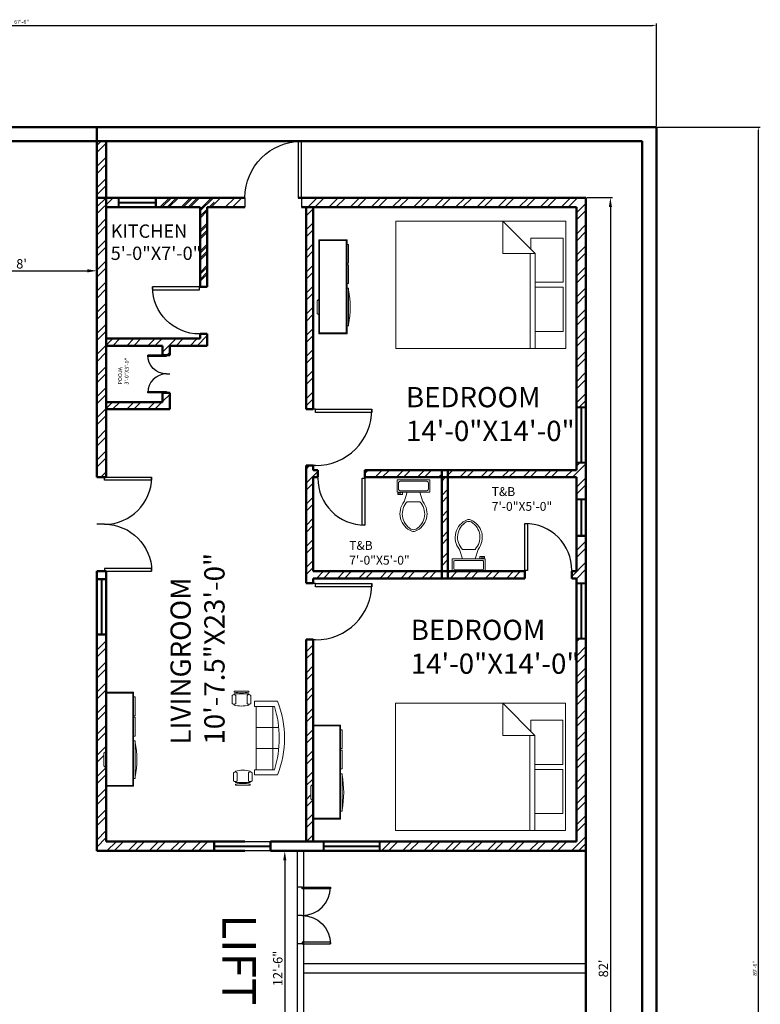
# Model space of a CAD drawing. Units: inches. Extents: x -12550 to 6516, y 1273 to 18700.
# Tile 15 of 19: x 4811 to 5284, y 1958 to 2587. Entities that reach past the tile are written whole.
import ezdxf

# ---------------------------------------------------------------- set-up
doc = ezdxf.new("R2010")
doc.units = ezdxf.units.IN
for name, color, linetype, lineweight in [('A-ANNO-DIMS', 2, 'Continuous', 18), ('A-AREA-IDEN', 1, 'Continuous', 18), ('A-DOOR', 5, 'Continuous', 25), ('A-EQPM', 4, 'Continuous', 25), ('A-FURN', 8, 'Continuous', 18), ('A-GLAZ', 3, 'Continuous', 25), ('A-WALL', 7, 'Continuous', 50), ('A-WALL-PATT', 8, 'Continuous', 13)]:
    doc.layers.add(name, color=color, linetype=linetype, lineweight=lineweight)
doc.styles.get("Standard").update_dxf_attribs({"font": 'arial.ttf'})
doc.dimstyles.new('ISO-25', dxfattribs={"dimtxt": 2.5, "dimasz": 2.5, "dimexe": 1.25, "dimexo": 0.625, "dimtad": 1, "dimlunit": 4, "dimtxsty": 'Standard', "dimcen": 2.5, "dimadec": 0, "dimazin": 0, "dimtfac": 1, "dimtmove": 0, "dimatfit": 3, "dimfxl": 1, "dimarcsym": 0})
pattern_1 = [(45, (2434.941, 0), (-6.735192, 6.735192), []), (45, (2439.432, 0), (-6.735192, 6.735192), [])]
pattern_2 = [(45, (2434.941, 567), (-6.735192, 6.735192), []), (45, (2439.432, 567), (-6.735192, 6.735192), [])]

# ---------------------------------------------------------------- blocks, each defined once
blk = doc.blocks.new('*U2')
for p, q in [((0, 0), (0, -5)), ((30, 0), (30, -5))]:
    blk.add_line(p, q)
blk.add_lwpolyline([(0, 0), (0, 30), (1.75, 30), (1.75, 0)], close=True)
blk.add_arc((0, 0), 30, 0, 90)
blk = doc.blocks.new('Bed - Queen')
for p, q in [((0, -80.00003), (0, 0)), ((0, 0), (59.99999, 0)), ((59.99999, 0), (59.99999, -80.00003)), ((7.99999, -1.2), (28.79998, -1.2)), ((7.99999, -14.4), (7.99999, -1.2)), ((28.79998, -1.2), (28.79998, -14.4)), ((31.19999, -1.2), (51.99999, -1.2)), ((31.19999, -14.4), (31.19999, -1.2)), ((51.99999, -1.2), (51.99999, -16.4)), ((0, -14.4), (44.8, -14.4)), ((44.8, -16.8), (0, -16.8)), ((59.99999, -29.6), (44.8, -14.4)), ((44.8, -14.4), (44.8, -29.6)), ((51.99999, -16.4), (46.79936, -16.4)), ((44.8, -29.6), (59.99999, -29.6)), ((59.99999, -80.00003), (0, -80.00003))]:
    blk.add_line(p, q)
blk = doc.blocks.new('Toilet - top')
for p, q in [((9.5, -6), (9.5, -2)), ((-10, -8.5), (-8, -8.5)), ((-10, -9.5), (-10, -8.5)), ((-7, -9.5), (-10, -9.5)), ((-8, -8.5), (-8, -8)), ((-7, -8), (-7, -9.5)), ((-4, -8), (-6, -14)), ((4, -8), (6, -14)), ((4, -14), (-4, -14))]:
    blk.add_line(p, q)
blk.add_lwpolyline([(10.5, -8), (10.5, 0), (-10.5, 0), (-10.5, -8)], close=True)
for points in [[(-9.5, -2), (-9.5, -6)], [(8.5, -1), (-8.5, -1)], [(-8.5, -7), (8.5, -7)]]:
    blk.add_lwpolyline(points)
for centre, radius, start, end in [((-8.62, -1.88), 0.884, 81.8699, 188.1301), ((-8.62, -6.12), 0.884, 171.8699, 278.1301), ((8.62, -1.88), 0.884, 351.8699, 98.1301), ((8.62, -6.12), 0.884, 261.8699, 8.1301), ((3.52, -21.58), 12.17, 141.46911, 247.97143), ((4.2, -21.82), 11.33, 136.36773, 238.94682), ((-3.52, -21.58), 12.17, 292.02843, 38.53071), ((-4.2, -21.82), 11.33, 301.05301, 43.63209), ((0, -27.88), 4, 245.73182, 294.26817), ((0, -29), 4, 254.86053, 285.13947)]:
    blk.add_arc(centre, radius, start, end)
blk = doc.blocks.new('Entertainment Center')
for p, q in [((-4, 0), (-5, -1)), ((4, 0), (-4, 0)), ((5, -1), (4, 0)), ((-17, -19), (-17, -1)), ((-17, -1), (43, -1)), ((-16.5, -18.5), (-16.5, -1.5)), ((-16.5, -1.5), (42.5, -1.5)), ((42.5, -1.5), (42.5, -18.5)), ((43, -1), (43, -19)), ((42.5, -18.5), (-16.5, -18.5)), ((43, -19), (-17, -19)), ((-12, -20), (-12, -19)), ((12, -20), (-12, -20)), ((12, -19), (12, -20)), ((15, -20), (15, -19)), ((27, -20), (15, -20)), ((27, -19), (27, -20)), ((28, -20), (28, -19)), ((40, -20), (28, -20)), ((40, -19), (40, -20))]:
    blk.add_line(p, q)
blk.add_arc((0, 40), 61, 259.6111, 280.3889)
blk = doc.blocks.new('Sofa - Roundback 7 ft.')
for p, q in [((-12.00002, -32.4421), (-12.00003, -6.5971)), ((11.99997, -32.4421), (11.99998, -6.5971)), ((-36.000027, -34), (-36.000027, -11.4696)), ((-35.999844, -13.3819), (35.9998, -13.3819)), ((35.99998, -34), (35.99998, -11.4696)), ((-36.000027, -32.4421), (35.99998, -32.4421))]:
    blk.add_line(p, q)
for points in [[(-36.000027, -34), (-42.000027, -34), (-42.000027, -8)], [(41.99998, -8), (41.99998, -34), (35.99998, -34)]]:
    blk.add_lwpolyline(points)
for centre, radius, start, end in [((0, -114.25), 114.25, 68.43141, 111.5686), ((-0.00001, -127.1968), 121.1968, 72.72033, 107.2797)]:
    blk.add_arc(centre, radius, start, end)
blk = doc.blocks.new('Chair - Desk')
for p, q in [((-8.5, 0), (-8.5, -1)), ((-8.5, 0), (8.5, 0)), ((8.5, 0), (8.5, -1)), ((-10.5, -5), (-10.5, -14)), ((-8.5, -3), (-8.5, -4)), ((-8.5, -3), (8.5, -3)), ((-6.5, -14), (-6.5, -5)), ((-2, -3), (-2, -1.9355)), ((2, -1.9576), (2, -3)), ((6.5, -5), (6.5, -14)), ((8.5, -3), (8.5, -4)), ((10.5, -14), (10.5, -5)), ((-8.5, -15), (-8.5, -16)), ((8.5, -15), (8.5, -16))]:
    blk.add_line(p, q)
for centre, radius, start, end in [((-8.5, -6.5), 2.5, 36.8699, 143.1301), ((0, 34.625), 36.625, 256.5803, 283.4197), ((8.5, -6.5), 2.5, 36.8699, 143.1301), ((-8.5, -12.5), 2.5, 216.8699, 323.1301), ((0, 19.625), 36.625, 256.5803, 283.4197), ((8.5, -12.5), 2.5, 216.8699, 323.1301)]:
    blk.add_arc(centre, radius, start, end)
blk = doc.blocks.new('*D40')
at = {"layer": 'A-ANNO-DIMS', "color": 0, "lineweight": -2, "transparency": 16777216}
for p, q in [((4988.01, 2056.25), (4979.29, 2056.25)), ((4980.54, 2050.25), (4980.54, 1912.25)), ((4988.01, 1906.25), (4979.29, 1906.25))]:
    blk.add_line(p, q, dxfattribs=at)
at = {"layer": 'A-ANNO-DIMS', "color": 0, "transparency": 16777216}
for points in [[(4979.54, 2050.25), (4981.54, 2050.25), (4980.54, 2056.25)], [(4979.54, 1912.25), (4981.54, 1912.25), (4980.54, 1906.25)]]:
    blk.add_solid(points, dxfattribs=at)
at = {"layer": 'Defpoints', "color": 0, "transparency": 16777216}
for p in [(4988.63, 2056.25), (4980.54, 1906.25), (4988.63, 1906.25)]:
    blk.add_point(p, dxfattribs=at)
at = {"layer": 'A-ANNO-DIMS', "color": 0, "transparency": 16777216, "insert": (4976.86, 1981.25), "char_height": 6, "attachment_point": 5, "rotation": 90}
blk.add_mtext('12\'-6"', dxfattribs=at)
blk = doc.blocks.new('*D42')
at = {"layer": 'A-ANNO-DIMS', "color": 0, "lineweight": -2, "transparency": 16777216}
for p, q in [((5173.26, 2473.25), (5189.5, 2473.25)), ((5188.25, 2467.25), (5188.25, 1495.25)), ((5173.26, 1489.25), (5189.5, 1489.25))]:
    blk.add_line(p, q, dxfattribs=at)
at = {"layer": 'A-ANNO-DIMS', "color": 0, "transparency": 16777216}
for points in [[(5187.25, 2467.25), (5189.25, 2467.25), (5188.25, 2473.25)], [(5187.25, 1495.25), (5189.25, 1495.25), (5188.25, 1489.25)]]:
    blk.add_solid(points, dxfattribs=at)
at = {"layer": 'Defpoints', "color": 0, "transparency": 16777216}
for p in [(5172.63, 2473.25), (5172.63, 1489.25), (5188.25, 1489.25)]:
    blk.add_point(p, dxfattribs=at)
at = {"layer": 'A-ANNO-DIMS', "color": 0, "transparency": 16777216, "insert": (5184.56, 1981.25), "char_height": 6, "attachment_point": 5, "rotation": 90}
blk.add_mtext("82'", dxfattribs=at)
blk = doc.blocks.new('*D39')
at = {"layer": 'A-ANNO-DIMS', "color": 0, "lineweight": -2, "transparency": 16777216}
for p, q in [((4764.63, 2407.12), (4764.63, 2427.81)), ((4770.63, 2426.56), (4854.63, 2426.56)), ((4860.63, 2407.12), (4860.63, 2427.81))]:
    blk.add_line(p, q, dxfattribs=at)
at = {"layer": 'A-ANNO-DIMS', "color": 0, "transparency": 16777216}
for points in [[(4770.63, 2427.56), (4770.63, 2425.56), (4764.63, 2426.56)], [(4854.63, 2427.56), (4854.63, 2425.56), (4860.63, 2426.56)]]:
    blk.add_solid(points, dxfattribs=at)
at = {"layer": 'Defpoints', "color": 0, "transparency": 16777216}
for p in [(4860.63, 2426.56), (4764.63, 2406.5), (4860.63, 2406.5)]:
    blk.add_point(p, dxfattribs=at)
at = {"layer": 'A-ANNO-DIMS', "color": 0, "transparency": 16777216, "insert": (4812.63, 2430.25), "char_height": 6, "attachment_point": 5}
blk.add_mtext("8'", dxfattribs=at)
blk = doc.blocks.new('WIN-3FT')
for p, q in [((0, 0), (0, 6)), ((0, 6), (36.02, 6)), ((36.02, 0), (0, 0)), ((0.5, 0), (0.5, 6)), ((35.52, 3.2), (0.5, 3.2)), ((35.52, 2.8), (0.5, 2.8)), ((35.52, 6), (35.52, 0)), ((36.02, 6), (36.02, 0))]:
    blk.add_line(p, q)
blk = doc.blocks.new('WIN-2FT')
for p, q in [((0, 0), (0, 24.02)), ((0, 24.02), (6, 24.02)), ((0, 23.52), (6, 23.52)), ((2.8, 0.5), (2.8, 23.52)), ((3.2, 0.5), (3.2, 23.52)), ((6, 24.02), (6, 0)), ((6, 0.5), (0, 0.5)), ((6, 0), (0, 0))]:
    blk.add_line(p, q)
blk = doc.blocks.new('*D112')
at = {"layer": 'A-ANNO-DIMS', "color": 0, "lineweight": -2, "transparency": 16777216}
for p, q in [((4407.63, 2518.87), (4407.63, 2584.5)), ((4410.13, 2583.25), (5215.13, 2583.25)), ((5217.63, 2518.87), (5217.63, 2584.5))]:
    blk.add_line(p, q, dxfattribs=at)
at = {"layer": 'A-ANNO-DIMS', "color": 0, "transparency": 16777216}
for points in [[(4410.13, 2583.66), (4410.13, 2582.83), (4407.63, 2583.25)], [(5215.13, 2583.66), (5215.13, 2582.83), (5217.63, 2583.25)]]:
    blk.add_solid(points, dxfattribs=at)
at = {"layer": 'Defpoints', "color": 0, "transparency": 16777216}
for p in [(5217.63, 2583.25), (4407.63, 2518.25), (5217.63, 2518.25)]:
    blk.add_point(p, dxfattribs=at)
at = {"layer": 'A-ANNO-DIMS', "color": 0, "transparency": 16777216, "insert": (4812.63, 2585.15), "char_height": 2.5, "attachment_point": 5}
blk.add_mtext('67\'-6"', dxfattribs=at)
blk = doc.blocks.new('*D113')
at = {"layer": 'A-ANNO-DIMS', "color": 0, "lineweight": -2, "transparency": 16777216}
for p, q in [((5218.26, 2518.25), (5283.88, 2518.25)), ((5282.63, 1446.75), (5282.63, 2515.75)), ((5218.26, 1444.25), (5283.88, 1444.25))]:
    blk.add_line(p, q, dxfattribs=at)
at = {"layer": 'A-ANNO-DIMS', "color": 0, "transparency": 16777216}
for points in [[(5282.21, 2515.75), (5283.05, 2515.75), (5282.63, 2518.25)], [(5282.21, 1446.75), (5283.05, 1446.75), (5282.63, 1444.25)]]:
    blk.add_solid(points, dxfattribs=at)
at = {"layer": 'Defpoints', "color": 0, "transparency": 16777216}
for p in [(5217.63, 2518.25), (5282.63, 2518.25), (5217.63, 1444.25)]:
    blk.add_point(p, dxfattribs=at)
at = {"layer": 'A-ANNO-DIMS', "color": 0, "transparency": 16777216, "insert": (5280.73, 1981.25), "char_height": 2.5, "attachment_point": 5, "rotation": 90}
blk.add_mtext('89\'-6"', dxfattribs=at)

msp = doc.modelspace()

# ---------------------------------------------------------------- hatches: boundary and pattern name
at = {"layer": 'A-WALL-PATT'}
h = msp.add_hatch(dxfattribs=at)
h.set_pattern_fill('ANSI32', color=256)
h.set_pattern_definition(pattern_1)
h.paths.add_polyline_path([(4866.63, 2509.247), (4860.63, 2509.247), (4860.63, 2473.247), (4866.63, 2473.247)])
h = msp.add_hatch(dxfattribs=at)
h.set_pattern_fill('ANSI32', color=256)
h.set_pattern_definition(pattern_2)
h.paths.add_polyline_path([(4874.387, 2473.247), (4860.63, 2473.247), (4860.63, 2294.747), (4865.63, 2294.747), (4866.63, 2294.747), (4866.63, 2467.247), (4874.387, 2467.247)])
h = msp.add_hatch(dxfattribs=at)
h.set_pattern_fill('ANSI32', color=256)
h.set_pattern_definition(pattern_1)
h.paths.add_polyline_path([(4898.405, 2473.247), (4898.405, 2467.247), (4926.63, 2467.247), (4926.63, 2416.247), (4931.13, 2416.247), (4931.13, 2467.247), (4955.13, 2467.247), (4955.13, 2473.247)])
h = msp.add_hatch(dxfattribs=at)
h.set_pattern_fill('ANSI32', color=256)
h.set_pattern_definition(pattern_2)
h.paths.add_polyline_path([(4935.469, 2473.247), (4898.405, 2473.247), (4898.405, 2467.247), (4926.63, 2467.247), (4926.63, 2416.247), (4931.13, 2416.247), (4931.13, 2467.247), (4935.469, 2467.247)])
h = msp.add_hatch(dxfattribs=at)
h.set_pattern_fill('ANSI32', color=256)
h.set_pattern_definition(pattern_2)
h.paths.add_polyline_path([(4991.13, 2473.247), (4991.13, 2467.247), (5166.63, 2467.247), (5166.63, 2339.747), (5172.63, 2339.747), (5172.63, 2473.247)])
h = msp.add_hatch(dxfattribs=at)
h.set_pattern_fill('ANSI32', color=256)
h.set_pattern_definition(pattern_2)
h.paths.add_polyline_path([(4998.63, 2467.247), (4994.13, 2467.247), (4994.13, 2338.247), (4998.63, 2338.247)])
h = msp.add_hatch(dxfattribs=at)
h.set_pattern_fill('ANSI32', color=256)
h.set_pattern_definition(pattern_2)
h.paths.add_polyline_path([(4931.13, 2386.247), (4926.63, 2386.247), (4926.63, 2383.247), (4866.63, 2383.247), (4866.63, 2378.747), (4902.63, 2378.747), (4902.63, 2372.747), (4905.13, 2372.747), (4907.13, 2372.747), (4907.13, 2378.747), (4931.13, 2378.747)])
h = msp.add_hatch(dxfattribs=at)
h.set_pattern_fill('ANSI32', color=256)
h.set_pattern_definition(pattern_2)
h.paths.add_polyline_path([(4907.13, 2348.747), (4905.13, 2348.747), (4902.63, 2348.747), (4902.63, 2342.747), (4866.63, 2342.747), (4866.63, 2338.247), (4907.13, 2338.247)])
h = msp.add_hatch(dxfattribs=at)
h.set_pattern_fill('ANSI32', color=256)
h.set_pattern_definition(pattern_2)
h.paths.add_polyline_path([(4998.63, 2294.747), (5001.63, 2294.747), (5001.63, 2299.247), (4998.63, 2299.247), (4998.63, 2302.247), (4994.13, 2302.247), (4994.13, 2227.247), (4998.63, 2227.247), (4998.63, 2230.247), (5001.583, 2230.247), (5080.63, 2230.247), (5080.63, 2234.747), (5001.583, 2234.747), (4998.63, 2234.747)])
h = msp.add_hatch(dxfattribs=at)
h.set_pattern_fill('ANSI32', color=256)
h.set_pattern_definition(pattern_2)
h.paths.add_polyline_path([(5172.63, 2303.73), (5166.63, 2303.73), (5166.63, 2299.247), (5163.63, 2299.247), (5084.63, 2299.247), (5084.63, 2294.747), (5163.63, 2294.747), (5166.63, 2294.747), (5166.63, 2281.042), (5172.63, 2281.042)])
h = msp.add_hatch(dxfattribs=at)
h.set_pattern_fill('ANSI32', color=256)
h.set_pattern_definition(pattern_2)
h.paths.add_polyline_path([(5080.63, 2299.247), (5031.63, 2299.247), (5031.63, 2294.747), (5080.63, 2294.747)], flags=17)
h = msp.add_hatch(dxfattribs=at)
h.set_pattern_fill('ANSI32', color=256)
h.set_pattern_definition(pattern_2)
h.paths.add_polyline_path([(5084.63, 2294.747), (5080.63, 2294.747), (5080.63, 2234.747), (5084.63, 2234.747)])
h = msp.add_hatch(dxfattribs=at)
h.set_pattern_fill('ANSI32', color=256)
h.set_pattern_definition(pattern_2)
h.paths.add_polyline_path([(5172.63, 2257.024), (5166.63, 2257.024), (5166.63, 2234.747), (5163.63, 2234.747), (5163.63, 2230.247), (5166.63, 2230.247), (5166.63, 2227.369), (5172.63, 2227.369)])
h = msp.add_hatch(dxfattribs=at)
h.set_pattern_fill('ANSI32', color=256)
h.set_pattern_definition(pattern_2)
h.paths.add_polyline_path([(5133.63, 2234.747), (5084.63, 2234.747), (5084.63, 2230.247), (5133.63, 2230.247)])
h = msp.add_hatch(dxfattribs=at)
h.set_pattern_fill('ANSI32', color=256)
h.set_pattern_definition(pattern_2)
h.paths.add_polyline_path([(4935.469, 2056.247), (4935.469, 2062.247), (4866.63, 2062.247), (4866.63, 2097.559), (4866.13, 2097.559), (4866.13, 2109.559), (4865.13, 2110.559), (4865.13, 2118.559), (4866.13, 2119.559), (4866.13, 2157.559), (4866.63, 2157.559), (4866.63, 2194.032), (4860.63, 2194.032), (4860.63, 2056.247)])
h = msp.add_hatch(dxfattribs=at)
h.set_pattern_fill('ANSI32', color=256)
h.set_pattern_definition(pattern_2)
h.paths.add_polyline_path([(4994.13, 2190.947), (4994.13, 2062.247), (4998.63, 2062.247), (4998.63, 2076.575), (4998.13, 2076.575), (4998.13, 2088.575), (4997.13, 2089.575), (4997.13, 2097.575), (4998.13, 2098.575), (4998.13, 2136.575), (4998.627, 2190.947)])
h = msp.add_hatch(dxfattribs=at)
h.set_pattern_fill('ANSI32', color=256)
h.set_pattern_definition(pattern_2)
h.paths.add_polyline_path([(5172.63, 2191.352), (5166.63, 2191.352), (5166.63, 2062.247), (5041.216, 2062.247), (5041.216, 2056.247), (5172.63, 2056.247)])

# ---------------------------------------------------------------- linework, layer by layer
at = {"layer": 'A-EQPM'}
for p, q in [((4988.63, 1906.247), (4988.63, 2056.247)), ((5172.63, 2056.247), (4988.63, 2056.247)), ((4992.63, 1906.247), (4992.63, 2056.247)), ((5172.63, 2056.247), (5172.63, 1906.247)), ((5172.63, 1984.247), (4992.63, 1984.247)), ((5172.63, 1978.247), (4992.63, 1978.247))]:
    msp.add_line(p, q, dxfattribs=at)
at = {"layer": 'A-WALL'}
for p, q in [((4407.63, 2518.247), (5217.63, 2518.247)), ((4860.63, 2294.747), (4860.63, 2518.247)), ((5217.63, 2518.247), (5217.63, 1444.247)), ((4416.63, 2509.247), (5208.63, 2509.247)), ((4989.03, 2509.247), (4689.03, 2509.247)), ((4866.63, 2294.747), (4866.63, 2509.247)), ((5208.63, 2509.247), (5208.63, 1453.247)), ((4955.13, 2473.247), (4860.63, 2473.247)), ((4994.13, 2473.247), (4989.03, 2473.247)), ((5172.63, 2473.247), (4994.13, 2473.247)), ((5172.63, 2060.923), (5172.63, 2473.247)), ((4926.63, 2467.247), (4866.63, 2467.247)), ((4926.63, 2416.247), (4926.63, 2467.247)), ((4955.13, 2467.247), (4931.13, 2467.247)), ((4931.13, 2416.247), (4931.13, 2467.247)), ((4994.13, 2467.247), (4991.13, 2467.247)), ((5166.63, 2467.247), (4994.13, 2467.247)), ((4994.13, 2338.247), (4994.13, 2467.247)), ((4998.63, 2338.247), (4998.63, 2467.247)), ((5166.63, 2299.247), (5166.63, 2467.247)), ((4926.63, 2416.247), (4931.13, 2416.247)), ((4926.63, 2383.247), (4866.63, 2383.247)), ((4926.63, 2383.247), (4926.63, 2386.247)), ((4931.13, 2386.247), (4926.63, 2386.247)), ((4931.13, 2378.747), (4931.13, 2386.247)), ((4931.13, 2383.247), (4931.13, 2386.247)), ((4902.63, 2378.747), (4866.63, 2378.747)), ((4902.63, 2372.747), (4902.63, 2378.747)), ((4931.13, 2378.747), (4907.13, 2378.747)), ((4907.13, 2372.747), (4907.13, 2378.747)), ((4902.63, 2372.747), (4907.13, 2372.747)), ((4902.63, 2342.747), (4902.63, 2348.747)), ((4907.13, 2348.747), (4902.63, 2348.747)), ((4907.13, 2338.247), (4907.13, 2348.747)), ((4907.13, 2342.747), (4907.13, 2348.747)), ((4902.63, 2342.747), (4866.63, 2342.747)), ((4907.13, 2338.247), (4866.63, 2338.247)), ((4994.13, 2338.247), (4998.63, 2338.247)), ((4994.13, 2227.247), (4994.13, 2302.247)), ((4998.63, 2302.247), (4994.13, 2302.247)), ((4998.63, 2299.247), (4998.63, 2302.247)), ((4998.63, 2299.247), (4998.63, 2302.247)), ((4998.63, 2299.247), (4998.63, 2302.247)), ((4998.63, 2299.247), (4998.63, 2302.247)), ((4866.63, 2294.747), (4860.63, 2294.747)), ((5001.63, 2299.247), (4998.63, 2299.247)), ((5001.63, 2294.747), (4998.63, 2294.747)), ((4998.63, 2234.747), (4998.63, 2294.747)), ((4998.63, 2234.747), (4998.63, 2294.747)), ((4998.63, 2234.747), (4998.63, 2294.747)), ((4998.63, 2294.747), (5001.63, 2294.747)), ((5001.63, 2294.747), (5001.63, 2299.247)), ((5163.63, 2299.247), (5031.63, 2299.247)), ((5031.63, 2299.247), (5031.63, 2294.747)), ((5163.63, 2294.747), (5031.63, 2294.747)), ((5080.63, 2230.247), (5080.63, 2299.247)), ((5084.63, 2230.247), (5084.63, 2299.247)), ((5166.63, 2299.247), (5163.63, 2299.247)), ((5166.63, 2299.247), (5163.63, 2299.247)), ((5166.63, 2294.747), (5163.63, 2294.747)), ((5166.63, 2234.747), (5166.63, 2294.747)), ((4866.63, 2234.747), (4860.63, 2234.747)), ((4860.63, 2056.247), (4860.63, 2234.747)), ((4866.63, 2062.247), (4866.63, 2234.747)), ((5001.583, 2234.747), (4998.63, 2234.747)), ((5133.63, 2234.747), (5001.583, 2234.747)), ((5133.63, 2234.747), (5133.63, 2230.247)), ((5166.63, 2234.747), (5163.63, 2234.747)), ((5163.63, 2230.247), (5163.63, 2234.747)), ((4994.13, 2230.247), (4994.13, 2227.247)), ((4994.13, 2227.247), (4998.63, 2227.247)), ((5001.583, 2230.247), (4998.63, 2230.247)), ((4998.63, 2227.247), (4998.63, 2230.247)), ((4998.63, 2227.247), (4998.63, 2230.247)), ((4998.63, 2227.247), (4998.63, 2230.247)), ((5133.63, 2230.247), (5001.583, 2230.247)), ((5166.63, 2230.247), (5163.63, 2230.247)), ((5166.63, 2230.247), (5163.63, 2230.247)), ((5166.63, 2062.247), (5166.63, 2230.247)), ((4994.13, 2062.247), (4994.13, 2191.247)), ((4998.63, 2191.247), (4994.13, 2191.247)), ((4998.63, 2062.247), (4998.63, 2191.247)), ((4955.13, 2062.247), (4866.63, 2062.247)), ((4935.469, 2062.247), (4935.469, 2056.247)), ((4971.486, 2062.247), (4971.486, 2056.247)), ((4991.13, 2062.247), (4971.486, 2062.247)), ((5166.63, 2062.247), (4991.13, 2062.247)), ((4994.13, 2062.247), (4991.13, 2062.247)), ((4955.13, 2056.247), (4860.63, 2056.247)), ((4971.486, 2056.247), (4991.13, 2056.247)), ((5172.63, 2056.247), (4991.13, 2056.247)), ((5172.63, 1489.247), (5172.63, 2060.923)), ((5208.63, 1489.247), (5208.63, 2060.923))]:
    msp.add_line(p, q, dxfattribs=at)

# ---------------------------------------------------------------- block references
at = {"layer": 'A-DOOR', "xscale": -1.199999999999999, "yscale": 1.199999999999999, "zscale": 1.199999999999999}
msp.add_blockref('*U2', (4991.13, 2473.247), dxfattribs=at)
at = {"layer": 'A-DOOR', "xscale": -1}
for p, rotation in [((4926.13, 2416.247), 90), ((4865.63, 2234.747), 270)]:
    msp.add_blockref('*U2', p, dxfattribs=dict(at, rotation=rotation))
at = {"layer": 'A-DOOR'}
for p, xscale, yscale, zscale, rotation in [((4905.13, 2372.747), -0.399999999999997, 0.399999999999997, 0.399999999999997, 90), ((4905.13, 2348.747), 0.399999999999997, 0.399999999999997, 0.399999999999997, 90.00000000000003), ((5000.13, 2338.247), 1.199999999999999, 1.199999999999999, 1.199999999999999, 270), ((5000.13, 2226.947), 1.199999999999999, 1.199999999999999, 1.199999999999999, 270)]:
    msp.add_blockref('*U2', p, dxfattribs=dict(at, xscale=xscale, yscale=yscale, zscale=zscale, rotation=rotation))
for p, rotation in [((4865.63, 2294.747), 270), ((5031.63, 2294.247), 180)]:
    msp.add_blockref('*U2', p, dxfattribs=dict(at, rotation=rotation))
msp.add_blockref('*U2', (5133.63, 2235.247), dxfattribs=at)
at = {"layer": 'A-EQPM', "yscale": 0.5999999999999954, "zscale": 0.5999999999999954, "rotation": 270}
for p, xscale in [((4991.63, 2033.042), 0.5999999999999954), ((4991.63, 1997.042), -0.5999999999999954)]:
    msp.add_blockref('*U2', p, dxfattribs=dict(at, xscale=xscale))
at = {"layer": 'A-FURN'}
for name, p, xscale, yscale, zscale, rotation in [('Bed - Queen', (5159.81, 2376.994), -1.354827908062564, 1.354827908062564, 1.354827908062564, 270), ('Sofa - Roundback 7 ft.', (4980.349, 2128.265), 0.5595223685495907, 0.5595223685495907, 0.5595223685495907, 270), ('Bed - Queen', (5159.649, 2069.217), -1.354827908062564, 1.354827908062564, 1.354827908062564, 270), ('Chair - Desk', (4953.764, 2098.281), 0.5595223685495907, 0.5595223685495907, 0.5595223685495907, 180)]:
    msp.add_blockref(name, p, dxfattribs=dict(at, xscale=xscale, yscale=yscale, zscale=zscale, rotation=rotation))
for name, p, rotation in [('Entertainment Center', (5001.26, 2403.379), 89.99999999999999), ('Toilet - top', (5097.899, 2234.747), 180), ('Entertainment Center', (4865.13, 2114.559), 89.99999999999999), ('Entertainment Center', (4997.13, 2093.575), 89.99999999999999)]:
    msp.add_blockref(name, p, dxfattribs=dict(at, rotation=rotation))
msp.add_blockref('Toilet - top', (5062.653, 2293.198), dxfattribs=at)
at = {"layer": 'A-FURN', "xscale": 0.5595223685495907, "yscale": 0.5595223685495907, "zscale": 0.5595223685495907}
msp.add_blockref('Chair - Desk', (4952.91, 2158.265), dxfattribs=at)
at = {"layer": 'A-GLAZ'}
for name, p, rotation in [('WIN-2FT', (4874.387, 2473.247), 269.9999999999974), ('WIN-3FT', (5172.63, 2303.73), 90.00000000000493), ('WIN-2FT', (5172.63, 2281.042), 180), ('WIN-3FT', (4866.63, 2194.032), 90.00000000000188), ('WIN-3FT', (5172.63, 2191.352), 90.00000000000468), ('WIN-3FT', (4971.486, 2062.247), 180), ('WIN-3FT', (5041.216, 2062.247), 180)]:
    msp.add_blockref(name, p, dxfattribs=dict(at, rotation=rotation))

# ---------------------------------------------------------------- texts
at = {"layer": 'A-AREA-IDEN', "attachment_point": 1}
for s, width, gutter_width, insert, char_height in [('KITCHEN\\P5\'-0"X7\'-0"', 1.29487, 42.422, (4869.51, 2456.124), 8.48435), ('T&B\\P7\'-0"X5\'-0"', 4.19569, 28.328, (5112.552, 2288.465), 5.66556), ('T&B\\P7\'-0"X5\'-0"', 4.19569, 28.328, (5021.643, 2254.107), 5.66556)]:
    msp.add_mtext_dynamic_manual_height_columns(s, width=width, gutter_width=gutter_width, heights=[0], dxfattribs=dict(at, insert=insert, char_height=char_height))
for s, width, gutter_width, insert, char_height, rotation in [('POOJA\\P3\'-0"X3\'-0"', 0.78585, 12.5, (4874.182, 2354.026), 2.5, 89.183853), ('LIFT', 3.27433, 107.272, (4962.118, 2015.823), 21.4543, 270)]:
    msp.add_mtext_dynamic_manual_height_columns(s, width=width, gutter_width=gutter_width, heights=[0], dxfattribs=dict(at, insert=insert, char_height=char_height, rotation=rotation))
at = {"layer": 'A-AREA-IDEN', "char_height": 12.93169, "attachment_point": 1}
for insert in [(5057.845, 2352.378), (5060.911, 2203.812)]:
    msp.add_mtext('BEDROOM\\P14\'-0"X14\'-0"', dxfattribs=dict(at, insert=insert))
at = {"layer": 'A-AREA-IDEN', "insert": (4907.654, 2124.153), "char_height": 12.93169, "attachment_point": 1, "rotation": 90}
msp.add_mtext('LIVINGROOM\\P10\'-7.5"X23\'-0"', dxfattribs=at)

# ---------------------------------------------------------------- dimensions: what is measured, and where the dimension line sits
at = {"layer": 'A-ANNO-DIMS'}
for base, p1, p2, override, picture, middle in [((5217.63, 2583.247), (4407.63, 2518.247), (5217.63, 2518.247), {"dimdec": 1, "dimlfac": 1, "dimrnd": 0, "dimzin": 1, "dimdsep": 46, "dimlunit": 4, "dimfrac": 2}, '*D112', (4812.63, 2585.149)), ((4860.63, 2426.562), (4764.63, 2406.497), (4860.63, 2406.497), {"dimtxt": 6, "dimasz": 6, "dimclrd": 0, "dimclre": 0, "dimclrt": 0}, '*D39', (4812.63, 2430.25))]:
    dim = msp.add_linear_dim(base=base, p1=p1, p2=p2, dimstyle='ISO-25', override=override, dxfattribs=at)
    dim.commit()
    dim.dimension.update_dxf_attribs({"geometry": picture, "text_midpoint": middle})
for base, p1, p2, override, picture, middle in [((5282.63, 2518.247), (5217.63, 1444.247), (5217.63, 2518.247), {"dimdec": 1, "dimlfac": 1, "dimrnd": 0, "dimzin": 1, "dimdsep": 46, "dimlunit": 4, "dimfrac": 2}, '*D113', (5280.729, 1981.247)), ((5188.25, 1489.247), (5172.63, 2473.247), (5172.63, 1489.247), {"dimtxt": 6, "dimasz": 6, "dimclrd": 0, "dimclre": 0, "dimclrt": 0}, '*D42', (5184.562, 1981.247)), ((4980.544, 1906.247), (4988.63, 2056.247), (4988.63, 1906.247), {"dimtxt": 6, "dimasz": 6, "dimclrd": 0, "dimclre": 0, "dimclrt": 0}, '*D40', (4976.855, 1981.247))]:
    dim = msp.add_linear_dim(base=base, p1=p1, p2=p2, angle=90, dimstyle='ISO-25', override=override, dxfattribs=at)
    dim.commit()
    dim.dimension.update_dxf_attribs({"geometry": picture, "text_midpoint": middle})

doc.saveas('drawing.dxf')
